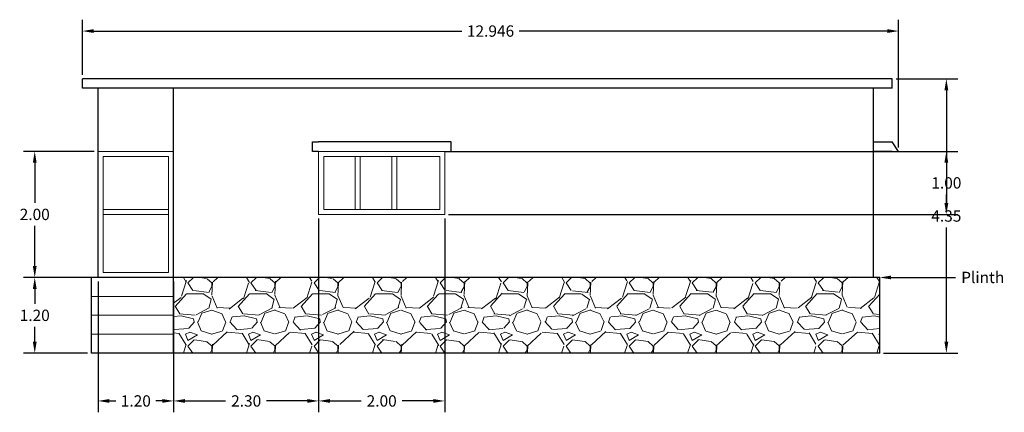
# Model space of a CAD drawing. Units: metres. Extents: x 37.9 to 70.9, y 22.7 to 44.8.
# Tile 3 of 4: x 38 to 53.6, y 38.6 to 44.8. Entities that reach past the tile are written whole.
import ezdxf
from ezdxf import colors
from ezdxf.entities.mleader import LeaderData, LeaderLine
from ezdxf.math import Vec2, Vec3

# ---------------------------------------------------------------- set-up
doc = ezdxf.new("R2010")
doc.units = ezdxf.units.M
doc.header["$LTSCALE"] = 50
doc.header["$MEASUREMENT"] = 0
doc.header["$PDMODE"] = 35
doc.header["$PDSIZE"] = -2
doc.linetypes.add('ACAD_ISO03W100', pattern=[30, 12, -18])
for name, color, linetype, lineweight in [('A-ANNO-DIMS', 2, 'Continuous', 18), ('A-ANNO-TEXT', 7, 'Continuous', 18), ('A-ELEV', 7, 'Continuous', 25), ('A-ELEV-DOOR', 4, 'Continuous', 18), ('A-ELEV-GLAZ', 4, 'Continuous', 18), ('A-ELEV-PATT', 8, 'Continuous', 13), ('A-ELEV-PLIN', 7, 'Continuous', 25), ('A-ELEV-ROOF', 7, 'Continuous', 25), ('A-ELEV-STRS', 7, 'Continuous', 18)]:
    doc.layers.add(name, color=color, linetype=linetype, lineweight=lineweight)
doc.styles.get("Standard").update_dxf_attribs({"font": 'arial.ttf'})
doc.dimstyles.get("Standard").update_dxf_attribs({"dimtxt": 0.18, "dimasz": 0.18, "dimexe": 0.18, "dimexo": 0.0625, "dimgap": 0.09, "dimtad": 0, "dimtih": 1, "dimtoh": 1, "dimzin": 0, "dimdsep": 46, "dimtxsty": 'Standard', "dimcen": 0.09, "dimadec": 0, "dimazin": 0, "dimtfac": 1, "dimtofl": 0, "dimtmove": 0, "dimatfit": 3, "dimfxl": 1, "dimtolj": 1, "dimtzin": 0, "dimarcsym": 0})

# ---------------------------------------------------------------- blocks, each defined once
blk = doc.blocks.new('*D34')
at = {"layer": 'A-ANNO-DIMS', "color": 0, "lineweight": -2, "transparency": 16777216}
for p, q in [((38.953604, 43.925786), (38.953604, 44.800786)), ((51.9, 42.775786), (51.9, 44.800786))]:
    blk.add_line(p, q, dxfattribs=at)
at = {"layer": 'A-ANNO-DIMS', "color": 0, "linetype": 'ACAD_ISO03W100', "lineweight": -2, "transparency": 16777216}
for p, q in [((39.133604, 44.620786), (44.97170650204638, 44.620786)), ((51.72, 44.620786), (45.8818974979536, 44.620786))]:
    blk.add_line(p, q, dxfattribs=at)
at = {"layer": 'A-ANNO-DIMS', "color": 0, "transparency": 16777216}
for points in [[(39.133604, 44.650786), (39.133604, 44.590786), (38.953604, 44.620786)], [(51.72, 44.650786), (51.72, 44.590786), (51.9, 44.620786)]]:
    blk.add_solid(points, dxfattribs=at)
at = {"layer": 'Defpoints', "color": 0, "transparency": 16777216}
for p in [(51.9, 44.620786), (38.953604, 43.863286), (51.9, 42.71328599999999)]:
    blk.add_point(p, dxfattribs=at)
at = {"layer": 'A-ANNO-DIMS', "color": 0, "transparency": 16777216, "insert": (45.42680199999999, 44.620786), "char_height": 0.18, "attachment_point": 5}
blk.add_mtext('\\A1;12.946', dxfattribs=at)
blk = doc.blocks.new('*D35')
at = {"layer": 'A-ANNO-DIMS', "color": 0, "lineweight": -2, "transparency": 16777216}
for p, q in [((51.86250000000002, 43.86328600000001), (52.83750000000005, 43.86328600000001)), ((51.66250000000003, 39.51328600000002), (52.83750000000005, 39.51328600000002))]:
    blk.add_line(p, q, dxfattribs=at)
at = {"layer": 'A-ANNO-DIMS', "color": 0, "linetype": 'ACAD_ISO03W100', "lineweight": -2, "transparency": 16777216}
for p, q in [((52.65750000000005, 43.68328600000001), (52.65750000000005, 41.87025052933153)), ((52.65750000000005, 39.69328600000002), (52.65750000000005, 41.5063214706685))]:
    blk.add_line(p, q, dxfattribs=at)
at = {"layer": 'A-ANNO-DIMS', "color": 0, "transparency": 16777216}
for points in [[(52.62750000000005, 43.68328600000001), (52.68750000000006, 43.68328600000001), (52.65750000000005, 43.86328600000001)], [(52.62750000000005, 39.69328600000002), (52.68750000000006, 39.69328600000002), (52.65750000000005, 39.51328600000002)]]:
    blk.add_solid(points, dxfattribs=at)
at = {"layer": 'Defpoints', "color": 0, "transparency": 16777216}
for p in [(51.80000000000003, 43.86328600000001), (52.65750000000005, 43.86328600000001), (51.60000000000003, 39.51328600000002)]:
    blk.add_point(p, dxfattribs=at)
at = {"layer": 'A-ANNO-DIMS', "color": 0, "transparency": 16777216, "insert": (52.65750000000005, 41.68828599999999), "char_height": 0.18, "attachment_point": 5}
blk.add_mtext('\\A1;4.35', dxfattribs=at)
blk = doc.blocks.new('*D36')
at = {"layer": 'A-ANNO-DIMS', "color": 0, "lineweight": -2, "transparency": 16777216}
for p, q in [((39.03428200000001, 40.71328600000001), (38.01610400000003, 40.71328600000001)), ((39.03428200000001, 39.51328600000002), (38.01610400000003, 39.51328600000002))]:
    blk.add_line(p, q, dxfattribs=at)
at = {"layer": 'A-ANNO-DIMS', "color": 0, "linetype": 'ACAD_ISO03W100', "lineweight": -2, "transparency": 16777216}
for p, q in [((38.19610400000003, 40.53328600000001), (38.19610400000003, 40.29518913778992)), ((38.19610400000003, 39.69328600000002), (38.19610400000003, 39.93138286221011))]:
    blk.add_line(p, q, dxfattribs=at)
at = {"layer": 'A-ANNO-DIMS', "color": 0, "transparency": 16777216}
for points in [[(38.16610400000003, 40.53328600000001), (38.22610400000003, 40.53328600000001), (38.19610400000003, 40.71328600000001)], [(38.16610400000003, 39.69328600000002), (38.22610400000003, 39.69328600000002), (38.19610400000003, 39.51328600000002)]]:
    blk.add_solid(points, dxfattribs=at)
at = {"layer": 'Defpoints', "color": 0, "transparency": 16777216}
for p in [(38.19610400000003, 40.71328600000001), (39.09678200000001, 40.71328600000001), (39.09678200000001, 39.51328600000002)]:
    blk.add_point(p, dxfattribs=at)
at = {"layer": 'A-ANNO-DIMS', "color": 0, "transparency": 16777216, "insert": (38.19610400000003, 40.113286), "char_height": 0.18, "attachment_point": 5}
blk.add_mtext('\\A1;1.20', dxfattribs=at)
blk = doc.blocks.new('*D37')
at = {"layer": 'A-ANNO-DIMS', "color": 0, "lineweight": -2, "transparency": 16777216}
for p, q in [((39.2, 40.65078599999999), (39.2, 38.575786)), ((40.4, 40.65078599999999), (40.4, 38.575786))]:
    blk.add_line(p, q, dxfattribs=at)
at = {"layer": 'A-ANNO-DIMS', "color": 0, "linetype": 'ACAD_ISO03W100', "lineweight": -2, "transparency": 16777216}
for p, q in [((39.38, 38.755786), (39.485, 38.755786)), ((40.22, 38.755786), (40.11499999999999, 38.755786))]:
    blk.add_line(p, q, dxfattribs=at)
at = {"layer": 'A-ANNO-DIMS', "color": 0, "transparency": 16777216}
for points in [[(39.38, 38.785786), (39.38, 38.725786), (39.2, 38.755786)], [(40.22, 38.785786), (40.22, 38.725786), (40.4, 38.755786)]]:
    blk.add_solid(points, dxfattribs=at)
at = {"layer": 'Defpoints', "color": 0, "transparency": 16777216}
for p in [(39.2, 40.713286), (40.4, 40.713286), (40.4, 38.755786)]:
    blk.add_point(p, dxfattribs=at)
at = {"layer": 'A-ANNO-DIMS', "color": 0, "transparency": 16777216, "insert": (39.8, 38.755786), "char_height": 0.18, "attachment_point": 5}
blk.add_mtext('\\A1;1.20', dxfattribs=at)
blk = doc.blocks.new('*D38')
at = {"layer": 'A-ANNO-DIMS', "color": 0, "lineweight": -2, "transparency": 16777216}
for p, q in [((42.7, 41.650786), (42.7, 38.575786)), ((40.4, 39.450786), (40.4, 38.575786))]:
    blk.add_line(p, q, dxfattribs=at)
at = {"layer": 'A-ANNO-DIMS', "color": 0, "linetype": 'ACAD_ISO03W100', "lineweight": -2, "transparency": 16777216}
for p, q in [((40.57999999999999, 38.755786), (41.22499317871759, 38.755786)), ((42.52, 38.755786), (41.8750068212824, 38.755786))]:
    blk.add_line(p, q, dxfattribs=at)
at = {"layer": 'A-ANNO-DIMS', "color": 0, "transparency": 16777216}
for points in [[(40.57999999999999, 38.785786), (40.57999999999999, 38.725786), (40.4, 38.755786)], [(42.52, 38.785786), (42.52, 38.725786), (42.7, 38.755786)]]:
    blk.add_solid(points, dxfattribs=at)
at = {"layer": 'Defpoints', "color": 0, "transparency": 16777216}
for p in [(42.7, 41.71328599999999), (40.4, 39.513286), (42.7, 38.755786)]:
    blk.add_point(p, dxfattribs=at)
at = {"layer": 'A-ANNO-DIMS', "color": 0, "transparency": 16777216, "insert": (41.55, 38.755786), "char_height": 0.18, "attachment_point": 5}
blk.add_mtext('\\A1;2.30', dxfattribs=at)
blk = doc.blocks.new('*D39')
at = {"layer": 'A-ANNO-DIMS', "color": 0, "lineweight": -2, "transparency": 16777216}
for p, q in [((42.7, 41.650786), (42.7, 38.575786)), ((44.7, 41.650786), (44.7, 38.575786))]:
    blk.add_line(p, q, dxfattribs=at)
at = {"layer": 'A-ANNO-DIMS', "color": 0, "linetype": 'ACAD_ISO03W100', "lineweight": -2, "transparency": 16777216}
for p, q in [((42.88, 38.755786), (43.3749931787176, 38.755786)), ((44.52, 38.755786), (44.0250068212824, 38.755786))]:
    blk.add_line(p, q, dxfattribs=at)
at = {"layer": 'A-ANNO-DIMS', "color": 0, "transparency": 16777216}
for points in [[(42.88, 38.785786), (42.88, 38.725786), (42.7, 38.755786)], [(44.52, 38.785786), (44.52, 38.725786), (44.7, 38.755786)]]:
    blk.add_solid(points, dxfattribs=at)
at = {"layer": 'Defpoints', "color": 0, "transparency": 16777216}
for p in [(42.7, 41.71328599999999), (44.7, 41.71328599999999), (44.7, 38.755786)]:
    blk.add_point(p, dxfattribs=at)
at = {"layer": 'A-ANNO-DIMS', "color": 0, "transparency": 16777216, "insert": (43.7, 38.755786), "char_height": 0.18, "attachment_point": 5}
blk.add_mtext('\\A1;2.00', dxfattribs=at)
blk = doc.blocks.new('*D40')
at = {"layer": 'A-ANNO-DIMS', "color": 0, "lineweight": -2, "transparency": 16777216}
for p, q in [((39.13750000000002, 42.71328600000001), (38.01610400000003, 42.71328600000001)), ((39.13750000000002, 40.71328600000001), (38.01610400000003, 40.71328600000001))]:
    blk.add_line(p, q, dxfattribs=at)
at = {"layer": 'A-ANNO-DIMS', "color": 0, "linetype": 'ACAD_ISO03W100', "lineweight": -2, "transparency": 16777216}
for p, q in [((38.19610400000003, 42.53328600000001), (38.19610400000003, 41.89518913778991)), ((38.19610400000003, 40.893286), (38.19610400000003, 41.5313828622101))]:
    blk.add_line(p, q, dxfattribs=at)
at = {"layer": 'A-ANNO-DIMS', "color": 0, "transparency": 16777216}
for points in [[(38.16610400000003, 42.53328600000001), (38.22610400000003, 42.53328600000001), (38.19610400000003, 42.71328600000001)], [(38.16610400000003, 40.893286), (38.22610400000003, 40.893286), (38.19610400000003, 40.71328600000001)]]:
    blk.add_solid(points, dxfattribs=at)
at = {"layer": 'Defpoints', "color": 0, "transparency": 16777216}
for p in [(38.19610400000003, 42.71328600000001), (39.20000000000002, 42.71328600000001), (39.20000000000002, 40.71328600000001)]:
    blk.add_point(p, dxfattribs=at)
at = {"layer": 'A-ANNO-DIMS', "color": 0, "transparency": 16777216, "insert": (38.19610400000003, 41.71328599999999), "char_height": 0.18, "attachment_point": 5}
blk.add_mtext('\\A1;2.00', dxfattribs=at)
blk = doc.blocks.new('*D41')
at = {"layer": 'A-ANNO-DIMS', "color": 0, "lineweight": -2, "transparency": 16777216}
for p, q in [((44.76250000000002, 42.71328600000001), (52.83750000000005, 42.71328600000002)), ((44.76250000000002, 41.71328600000001), (52.83750000000005, 41.71328600000001))]:
    blk.add_line(p, q, dxfattribs=at)
at = {"layer": 'A-ANNO-DIMS', "color": 0, "linetype": 'ACAD_ISO03W100', "lineweight": -2, "transparency": 16777216}
for p, q in [((52.65750000000005, 42.53328600000002), (52.65750000000005, 42.39518913778992)), ((52.65750000000005, 41.89328600000002), (52.65750000000005, 42.03138286221011))]:
    blk.add_line(p, q, dxfattribs=at)
at = {"layer": 'A-ANNO-DIMS', "color": 0, "transparency": 16777216}
for points in [[(52.62750000000005, 42.53328600000002), (52.68750000000006, 42.53328600000002), (52.65750000000005, 42.71328600000002)], [(52.62750000000005, 41.89328600000002), (52.68750000000006, 41.89328600000002), (52.65750000000005, 41.71328600000001)]]:
    blk.add_solid(points, dxfattribs=at)
at = {"layer": 'Defpoints', "color": 0, "transparency": 16777216}
for p in [(44.70000000000001, 42.71328600000001), (52.65750000000005, 42.71328600000002), (44.70000000000001, 41.71328600000001)]:
    blk.add_point(p, dxfattribs=at)
at = {"layer": 'A-ANNO-DIMS', "color": 0, "transparency": 16777216, "insert": (52.65750000000005, 42.21328599999999), "char_height": 0.18, "attachment_point": 5}
blk.add_mtext('\\A1;1.00', dxfattribs=at)

msp = doc.modelspace()

# ---------------------------------------------------------------- hatches: boundary and pattern name
at = {"layer": 'A-ELEV-PATT'}
h = msp.add_hatch(dxfattribs=at)
h.set_pattern_fill('GRAVEL', color=256)
h.set_pattern_definition([(228.012787504, (0.72, 1), (-8.000000000000062, -9.000000000000004), [0.134536, -13.3190880470737]), (184.969740728, (0.63, 0.9), (11.99999999999997, 1.000000000000035), [0.230868, -22.85592476122999]), (132.510447078, (0.4, 0.88), (10.00000000000011, -10.99999999999986), [0.162788, -16.1160325960997]), (267.273689006, (0.01, 0.63), (1.000000000000024, 20.00000000000002), [0.210238, -20.813558041629]), (292.833654178, (0, 0.4200000000000001), (-4.999999999999988, 12.00000000000003), [0.2061549999999999, -20.4093731280883]), (357.273689006, (0.08, 0.23), (-20.00000000000002, 1.000000000000025), [0.210238, -20.813558041629]), (37.6942404667, (0.29, 0.22), (-13, -9.999999999999973), [0.278029, -27.524848548916]), (72.2553283749, (0.51, 0.39), (7.000000000000027, 22.00000000000001), [0.2624879999999999, -25.9863214968134]), (121.429565615, (0.59, 0.6400000000000001), (-8.00000000000002, 12.99999999999999), [0.21095, -20.884073109729]), (175.236358309, (0.48, 0.82), (10.99999999999998, -1.000000000000037), [0.240832, -11.8007625787923]), (222.397437798, (0.24, 0.84), (-11.99999999999996, -10.99999999999997), [0.311448, -30.8333750047949]), (138.814074834, (1, 0.6200000000000001), (-7.000000000000032, 6), [0.106301, -10.52384481273469]), (171.46923439, (0.9200000000000002, 0.69), (13, -1.999999999999995), [0.202237, -20.021511416157]), (225, (0.72, 0.72), (-1e-16, -0.9999999999999328), [0.141421, -1.2727925623731]), (203.198590514, (0.65, 0.84), (4.999999999999989, 1.999999999999975), [0.076158, -7.5396151058639]), (291.801409486, (0.58, 0.81), (-0.9999999999996839, 3.000000000000102), [0.107703, -5.2774618071345]), (30.96375653209999, (0.6200000000000001, 0.71), (3.000000000000053, 1.999999999999979), [0.174929, -5.656022894845299]), (161.565051177, (0.7700000000000001, 0.8), (2.000000000000011, -0.9999999999999767), [0.126491, -3.035786660168399]), (16.389540334, (0, 0.81), (9.999999999999966, 3.000000000000043), [0.1772, -17.5428451466694]), (70.3461759419, (0.17, 0.8599999999999999), (-4.00000000000122, -11.00000000000339), [0.148661, -14.717407747319]), (293.198590514, (0.7700000000000001, 1), (-1.99999999999997, 4.999999999999991), [0.152315, -7.4634581058639]), (343.610459666, (0.8299999999999998, 0.8599999999999999), (-9.999999999999966, 3.000000000000043), [0.1772, -17.54284514666899]), (339.44395478, (0, 0.19), (-5.000000000000036, 2.000000000000024), [0.17088, -8.373123745317498]), (294.775140569, (0.16, 0.13), (-5.000000000000005, 11), [0.143178, -14.174643063276]), (66.8014094864, (0.7800000000000001, 0), (1.999999999999981, 4.999999999999969), [0.152315, -7.4634581058639]), (17.3540246363, (0.84, 0.14), (-12.99999999999998, -3.999999999999962), [0.167631, -16.59542361424]), (69.4439547804, (0.29, 0), (-2.000000000000007, -4.999999999999954), [0.08544, -8.458563745317498]), (101.309932474, (0.72, 0), (-0.9999999999999637, 4.000000000000012), [0.05099, -5.048029513592799]), (165.963756532, (0.71, 0.05), (2.999999999999958, -1.000000000000001), [0.206155, -3.9169506256177]), (186.009005957, (0.51, 0.1), (10.00000000000004, 0.9999999999999831), [0.19105, -18.9139231745428]), (303.690067526, (0.6200000000000001, 0.6200000000000001), (-0.9999999999999872, 1.999999999999985), [0.144222, -3.461329275463999]), (353.157226587, (0.7, 0.5), (17.00000000000001, -2.000000000000052), [0.251794, -24.9275626240283]), (60.9453959009, (0.95, 0.47), (-3.999999999999975, -6.999999999999976), [0.102956, -10.192674140987]), (90, (1, 0.56), (-0.9999999999999998, 1), [0.06, -0.9399999999999998]), (120.256437164, (0.4900000000000001, 0.13), (4.000000000000008, -7.000000000000007), [0.138924, -13.7535199894498]), (48.01278750419999, (0.4200000000000001, 0.25), (8, 8.999999999999975), [0.269072, -13.1845520470737]), (0, (0.6, 0.45), (1, 1), [0.26, -0.7400000000000001]), (325.304846469, (0.8599999999999999, 0.45), (10.00000000000014, -6.999999999999825), [0.158114, -15.653274300842]), (254.0546040990001, (0.99, 0.36), (-1.000000000000037, -4.000000000000004), [0.145602, -7.1345078892805]), (207.645975364, (0.95, 0.22), (-18.99999999999995, -10.00000000000005), [0.237065, -23.4694741822594]), (175.42607874, (0.7400000000000001, 0.11), (-12.99999999999995, 1.000000000000001), [0.250799, -24.8290734079689])])
h.paths.add_polyline_path([(40.39999999999999, 40.71328566870795), (40.39999999999999, 39.51328566870797), (51.6, 39.51328566870797), (51.6, 40.71328566870795)])

# ---------------------------------------------------------------- linework, layer by layer
at = {"layer": 'A-ELEV'}
for p, q in [((39.2, 40.71328566870795), (39.2, 43.71328566870795)), ((40.39999999999999, 39.51328566870797), (40.39999999999999, 43.71328566870795)), ((51.49999999999999, 40.71328566870795), (51.49999999999999, 43.71328566870795))]:
    msp.add_line(p, q, dxfattribs=at)
at = {"layer": 'A-ELEV-DOOR'}
for p, q in [((40.39999999999998, 42.71328566870795), (39.2, 42.71328566870795)), ((40.31999999999999, 41.79328566870794), (39.28, 41.79328566870795)), ((40.31999999999999, 41.71328566870794), (39.28, 41.71328566870795))]:
    msp.add_line(p, q, dxfattribs=at)
for points in [[(39.2, 40.71328566870795), (40.39999999999999, 40.71328566870795), (40.39999999999999, 42.71328566870795), (39.2, 42.71328566870795)], [(39.28, 40.79328566870795), (40.31999999999999, 40.79328566870795), (40.31999999999999, 42.63328566870796), (39.28, 42.63328566870796)]]:
    msp.add_lwpolyline(points, close=True, dxfattribs=at)
at = {"layer": 'A-ELEV-GLAZ'}
for p, q in [((42.78000000000001, 41.79328566870794), (42.78000000000001, 42.63328566870796)), ((42.78000000000001, 42.63328566870796), (44.62000000000001, 42.63328566870796)), ((43.28000000000001, 41.79328566870794), (43.28000000000001, 42.63328566870796)), ((43.36000000000001, 41.79328566870794), (43.36000000000001, 42.63328566870796)), ((43.86000000000001, 41.79328566870794), (43.86000000000001, 42.63328566870796)), ((43.94000000000001, 41.79328566870794), (43.94000000000001, 42.63328566870796)), ((44.62000000000001, 42.63328566870796), (44.61999999999999, 41.79328566870796)), ((44.61999999999999, 41.79328566870796), (42.78000000000001, 41.79328566870794))]:
    msp.add_line(p, q, dxfattribs=at)
msp.add_lwpolyline([(44.69999999999999, 41.71328566870796), (42.70000000000001, 41.71328566870794), (42.70000000000001, 42.71328566870796), (44.70000000000001, 42.71328566870795)], close=True, dxfattribs=at)
at = {"layer": 'A-ELEV-PLIN'}
for p, q in [((51.6, 40.71328566870795), (39.09678210177316, 40.71328566870795)), ((39.09678210177316, 39.51328566870797), (39.09678210177316, 40.71328566870795)), ((51.6, 39.51328566870797), (51.6, 40.71328566870795)), ((51.59999999999999, 39.51328566870797), (39.09678210177316, 39.51328566870797)), ((51.59999999999999, 39.51328566870797), (39.09678210177316, 39.51328566870797)), ((51.59999999999999, 39.51328566870797), (39.09678210177316, 39.51328566870797)), ((51.59999999999999, 39.51328566870797), (39.09678210177316, 39.51328566870797)), ((51.59999999999999, 39.51328566870797), (39.09678210177316, 39.51328566870797))]:
    msp.add_line(p, q, dxfattribs=at)
at = {"layer": 'A-ELEV-ROOF'}
for p, q in [((38.95360350875367, 43.71328566870794), (38.95360350875367, 43.86328566870795)), ((51.79999999999999, 43.86328566870796), (38.95360350875367, 43.86328566870794)), ((51.79999999999999, 43.71328566870795), (51.79999999999999, 43.86328566870796)), ((51.6, 43.71328566870795), (38.95360350875367, 43.71328566870795)), ((44.90000000000001, 43.71328566870795), (42.50000000000001, 43.71328566870794)), ((51.79999999999999, 43.71328566870795), (51.49999999999999, 43.71328566870795)), ((42.6, 42.71328566870796), (42.6, 42.86328566870795)), ((42.6, 42.86328566870795), (42.70000000000001, 42.86328566870795)), ((44.80000000000001, 42.86328566870794), (42.70000000000001, 42.86328566870795)), ((44.80000000000001, 42.71328566870795), (44.80000000000001, 42.86328566870795)), ((51.49999999999999, 42.86328566870795), (51.79999999999999, 42.86328566870795)), ((51.89999999999999, 42.71328566870796), (51.79999999999999, 42.86328566870795)), ((42.70000000000001, 42.71328566870796), (42.6, 42.71328566870796)), ((44.70000000000001, 42.71328566870795), (44.80000000000001, 42.71328566870795)), ((51.79999999999999, 42.71328566870796), (51.49999999999998, 42.71328566870796)), ((51.79999999999999, 42.71328566870796), (51.89999999999999, 42.71328566870796))]:
    msp.add_line(p, q, dxfattribs=at)
at = {"layer": 'A-ELEV-STRS'}
for p, q in [((40.39999999999999, 40.41328566870796), (39.09678210177316, 40.41328566870796)), ((40.39999999999999, 40.11328566870796), (39.09678210177316, 40.11328566870796)), ((40.39999999999999, 39.81328566870796), (39.09678210177316, 39.81328566870796))]:
    msp.add_line(p, q, dxfattribs=at)

# ---------------------------------------------------------------- dimensions: what is measured, and where the dimension line sits
at = {"layer": 'A-ANNO-DIMS'}
for base, p1, p2, override, picture, middle in [((51.9, 44.620786), (38.953604, 43.863286), (51.9, 42.71328599999999), {"dimdec": 3, "dimlfac": 1, "dimrnd": 0, "dimzin": 0, "dimdsep": 46, "dimlunit": 2}, '*D34', (45.42680199999999, 44.620786)), ((42.7, 38.755786), (40.4, 39.513286), (42.7, 41.71328599999999), {"dimdec": 2, "dimlfac": 1, "dimrnd": 0, "dimzin": 0, "dimdsep": 46, "dimlunit": 2}, '*D38', (41.55, 38.755786)), ((44.7, 38.755786), (42.7, 41.71328599999999), (44.7, 41.71328599999999), {"dimdec": 2, "dimlfac": 1, "dimrnd": 0, "dimzin": 0, "dimdsep": 46, "dimlunit": 2}, '*D39', (43.7, 38.755786)), ((40.4, 38.755786), (39.2, 40.713286), (40.4, 40.713286), {"dimdec": 2, "dimlfac": 1, "dimrnd": 0, "dimzin": 0, "dimdsep": 46, "dimlunit": 2}, '*D37', (39.8, 38.755786))]:
    dim = msp.add_linear_dim(base=base, p1=p1, p2=p2, dimstyle='Standard', override=override, dxfattribs=at)
    dim.commit()
    dim.dimension.update_dxf_attribs({"geometry": picture, "text_midpoint": middle})
for base, p1, p2, picture, middle in [((52.65750000000005, 43.86328600000001), (51.6, 39.513286), (51.79999999999999, 43.863286), '*D35', (52.65750000000005, 41.68828599999999)), ((38.19610400000003, 42.71328600000001), (39.2, 40.713286), (39.2, 42.71328599999999), '*D40', (38.19610400000003, 41.71328599999999)), ((52.65750000000005, 42.71328600000002), (44.7, 41.71328599999999), (44.7, 42.71328599999999), '*D41', (52.65750000000005, 42.21328599999999)), ((38.19610400000003, 40.71328600000001), (39.096782, 39.513286), (39.096782, 40.713286), '*D36', (38.19610400000003, 40.113286))]:
    dim = msp.add_linear_dim(base=base, p1=p1, p2=p2, angle=90, dimstyle='Standard', override={"dimdec": 2, "dimlfac": 1, "dimrnd": 0, "dimzin": 0, "dimdsep": 46, "dimlunit": 2}, dxfattribs=at)
    dim.commit()
    dim.dimension.update_dxf_attribs({"geometry": picture, "text_midpoint": middle})

# ---------------------------------------------------------------- leaders
at = {"layer": 'A-ANNO-TEXT'}
ml = msp.add_multileader_mtext('Standard', dxfattribs=at)
ml.set_content('Plinth', color=256)
ml.set_leader_properties()
ml.build(insert=Vec2(0, 0))
ml.multileader.update_dxf_attribs({"dogleg_length": 0.36, "arrow_head_size": 0.18})
ctx = ml.context
ctx.base_point, ctx.char_height, ctx.arrow_head_size, ctx.landing_gap_size, ctx.plane_origin = Vec3(52.80276103255035, 40.71328566870795), 0.18, 0.18, 0.09, Vec3(51.6, 40.71328566870795)
notes = []
notes.append((ctx, [(0, (1, 1, 0), (52.44276103255035, 40.71328566870795), (1, 0), 0.36, [(0, [(51.6, 40.71328566870795)], 0, [])])]))
ctx.mtext.insert, ctx.mtext.flow_direction = Vec3(52.89276103255035, 40.8041451502905), 5
for ctx, leaders in notes:
    for number, flags, end, landing, length, lines in leaders:
        leader = LeaderData()
        leader.index, (leader.has_last_leader_line, leader.has_dogleg_vector, leader.attachment_direction) = number, flags
        leader.last_leader_point, leader.dogleg_vector, leader.dogleg_length = Vec3(end), Vec3(landing), length
        for number, points, colour, breaks in lines:
            line = LeaderLine()
            line.index, line.vertices, line.color, line.breaks = number, Vec3.list(points), colors.encode_raw_color(colour), breaks
            leader.lines.append(line)
        ctx.leaders.append(leader)

doc.saveas('drawing.dxf')
